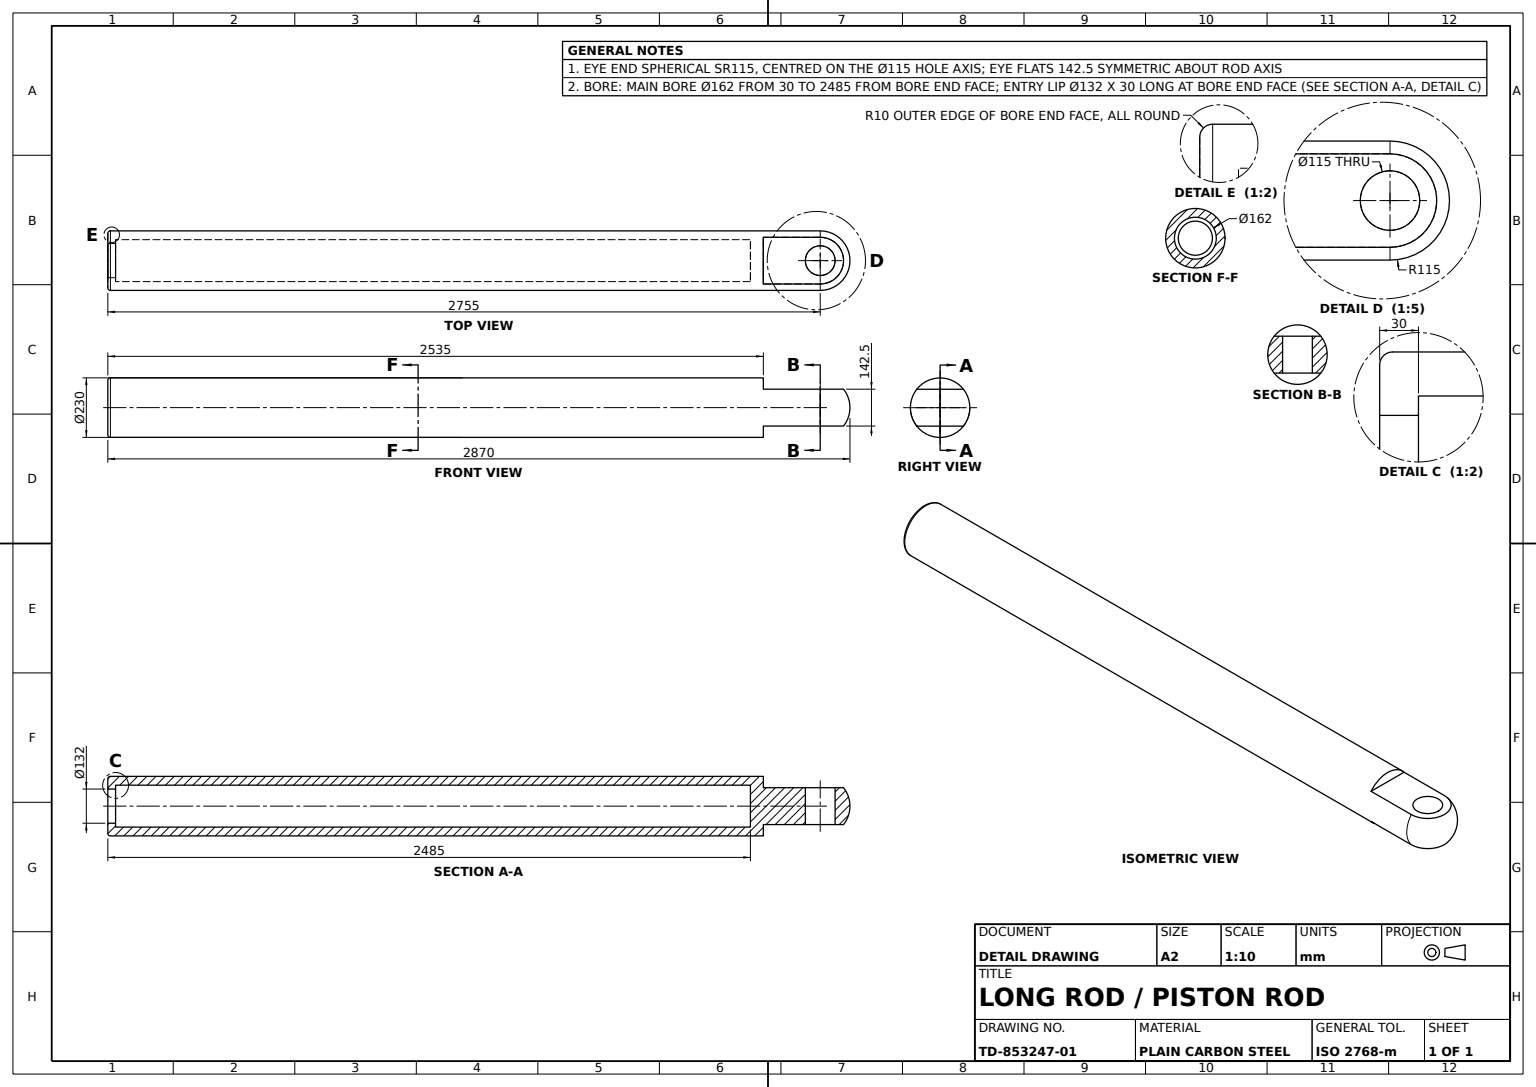
from build123d import *

# Parameters (mm, degrees)
BARREL_PROFILE_230_SKETCH_R  = 115
BARREL_BODY_230X2900_DEPTH   = 1450
END_TRIM_CUT_SKETCH_R        = 57.49999999999997
END_TRIM_CUT_DEPTH           = 1450
CLEVIS_EYE_PROFILE_SKETCH_W  = 365
CLEVIS_EYE_PROFILE_SKETCH_H  = 180.83378269641366
CLEVIS_EYE_PROFILE_CUT_DEPTH = 1450
EDGE_FILLET_R10_R            = 10


with BuildPart() as part:
    # Barrel Profile Ø230 Sketch → Barrel Body Ø230x2900 (new, symmetric)
    with BuildSketch(Plane.XY):
        Circle(BARREL_PROFILE_230_SKETCH_R)
    extrude(amount=BARREL_BODY_230X2900_DEPTH, both=True)

    # End Trim Cut Sketch → End Trim Cut (cut, symmetric)
    with BuildSketch(Plane(origin=(0, 0, 0), x_dir=(1, 0, 0), z_dir=(0, 1, 0))):
        with Locations(Location((0, 1305, 0), (0, 0, 270))):
            Circle(END_TRIM_CUT_SKETCH_R)
    extrude(amount=END_TRIM_CUT_DEPTH, both=True, mode=Mode.SUBTRACT)

    # Clevis Eye Profile Sketch → Clevis Eye Profile Cut (cut, symmetric)
    with BuildSketch(Plane(origin=(0, 0, 0), x_dir=(0, 0, -1), z_dir=(1, 0, 0))):
        with Locations((1267.5, -161.66689134820675)):
            Rectangle(CLEVIS_EYE_PROFILE_SKETCH_W, CLEVIS_EYE_PROFILE_SKETCH_H)
        with Locations((1267.5, 161.66689134820675)):
            Rectangle(CLEVIS_EYE_PROFILE_SKETCH_W, CLEVIS_EYE_PROFILE_SKETCH_H)
    extrude(amount=CLEVIS_EYE_PROFILE_CUT_DEPTH, both=True, mode=Mode.SUBTRACT)

    # Bore End Revolve Sketch → Bore End Revolved Cut (revolve, cut)
    with BuildSketch(Plane(origin=(0, 0, 0), x_dir=(1, 0, 0), z_dir=(0, 1, 0)), mode=Mode.PRIVATE) as bore_end_revolved_cut_sk:
        with BuildLine():
            Line((0, 1537.1393692003157), (209.05243850437193, 1537.1393692003157))
            Line((209.05243850437193, 1537.1393692003157), (209.05243850437193, 1305))
            Line((209.05243850437193, 1305), (115, 1305))
            ThreePointArc((115, 1305), (81.31727983645297, 1386.317279836453), (0, 1420))
            Line((0, 1420), (0, 1537.1393692003157))
        make_face()
    revolve(bore_end_revolved_cut_sk.sketch.rotate(Axis((0, 0, -1420), (0, 0, -1)), 218.284391292), axis=Axis((0, 0, -1420), (0, 0, -1)), mode=Mode.SUBTRACT)

    # Eye End Revolve Sketch → Eye End Revolved Cut (revolve, cut)
    with BuildSketch(Plane(origin=(0, 0, 0), x_dir=(1, 0, 0), z_dir=(0, 1, 0))):
        Polygon((0, -1450), (-6.94e-15, 1034.9999999999995), (81, 1035), (81, -1420), (66, -1420), (66, -1450), align=None)
    revolve(axis=Axis((0, 0, 1450), (0, 0, -1)), mode=Mode.SUBTRACT)

    # Edge Fillet R10
    edge_fillet_r10_edges = [part.edges().sort_by_distance(p)[0] for p in [
        (-115, 1.408e-14, 1450),
    ]]
    fillet(edge_fillet_r10_edges, radius=EDGE_FILLET_R10_R)


solid = part.part
